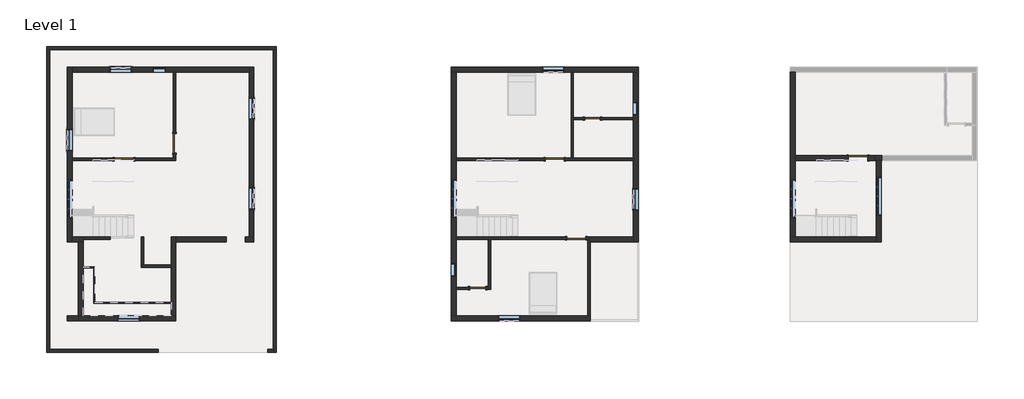
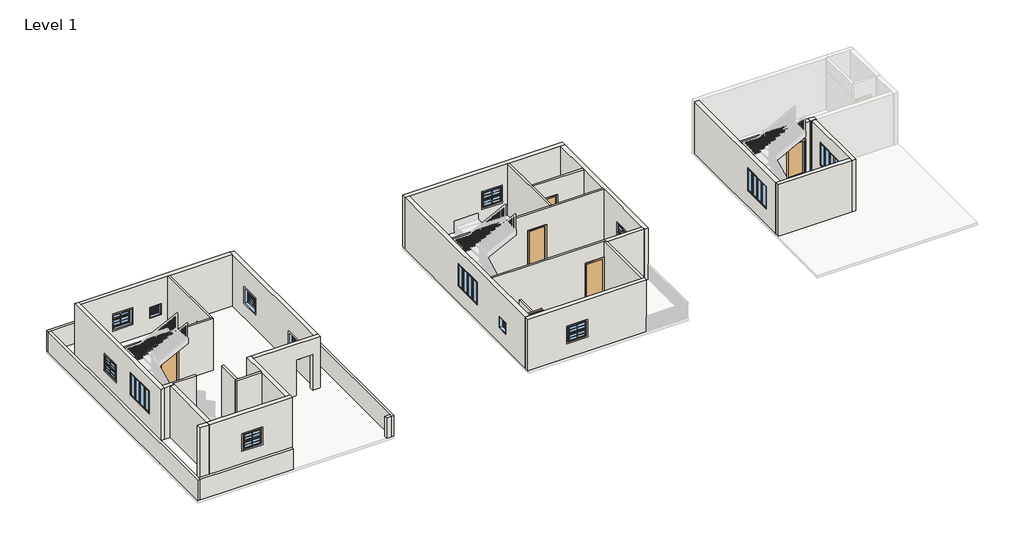
# One storey, part 1 of 8: 40 walls, 15 windows, 7 doors.
# Revit data of these elements (continued)
# Element 51 (IfcWindow, "Window-Awning-Double-Vertical : 41\" x 36\"")
#   Mark = "8"
#   Window Inset = 0' - 0"
#   Interior Wall Closure = 0' - 2 1/4"
#   Frame Extension = 0' - 0 1/4"
#   Exterior Wall Closure = 0' - 1 1/4"
#   Interior Trim Visibility = yes
#   Exterior Trim Visibility = yes
#   Phase Created = New Construction
#   Materials on its faces: "Wood - Stained", "Glass", "Clad - White"
# Element 52 (IfcWindow, "Window-Awning-Double-Vertical : 41\" x 36\"")
#   Mark = "9"
#   Window Inset = 0' - 0"
#   Interior Wall Closure = 0' - 2 1/4"
#   Frame Extension = 0' - 0 1/4"
#   Exterior Wall Closure = 0' - 1 1/4"
#   Interior Trim Visibility = yes
#   Exterior Trim Visibility = yes
#   Phase Created = New Construction
#   Materials on its faces: "Wood - Stained", "Glass", "Clad - White"
# Element 53 (IfcWindow, "Window-Awning-Double-Vertical : 41\" x 36\"")
#   Mark = "10"
#   Window Inset = 0' - 0"
#   Interior Wall Closure = 0' - 2 1/4"
#   Frame Extension = 0' - 0 1/4"
#   Exterior Wall Closure = 0' - 1 1/4"
#   Interior Trim Visibility = yes
#   Exterior Trim Visibility = yes
#   Phase Created = New Construction
#   Materials on its faces: "Wood - Stained", "Glass", "Clad - White"
# Element 54 (IfcWindow, "Window-Awning-Double-Vertical : 41\" x 36\"")
#   Mark = "11"
#   Window Inset = 0' - 0"
#   Interior Wall Closure = 0' - 2 1/4"
#   Frame Extension = 0' - 0 1/4"
#   Exterior Wall Closure = 0' - 1 1/4"
#   Interior Trim Visibility = yes
#   Exterior Trim Visibility = yes
#   Phase Created = New Construction
#   Materials on its faces: "Wood - Stained", "Glass", "Clad - White"
# Element 55 (IfcWindow, "Window-Awning-Double-Vertical : 41\" x 36\"")
#   Mark = "12"
#   Window Inset = 0' - 0"
#   Interior Wall Closure = 0' - 2 1/4"
#   Frame Extension = 0' - 0 1/4"
#   Exterior Wall Closure = 0' - 1 1/4"
#   Interior Trim Visibility = yes
#   Exterior Trim Visibility = yes
#   Phase Created = New Construction
#   Materials on its faces: "Wood - Stained", "Glass", "Clad - White"
# Element 56 (IfcWindow, "Window-Casement-Multi-Sash-Horizontal : 72\" x 53\"")
#   Mark = "1"
#   Window Inset = 0' - 0 5/8"
#   Frame Gap 3 = 0' - 1 83/128"
#   Frame Gap 2 = 0' - 0 5/8"
#   Phase Created = New Construction
#   Materials on its faces: "Metal - Aluminum", "Glass"
# Element 57 (IfcWindow, "Window-Casement-Multi-Sash-Horizontal : 72\" x 53\"")
#   Mark = "2"
#   Window Inset = 0' - 0 5/8"
#   Frame Gap 3 = 0' - 1 83/128"
#   Frame Gap 2 = 0' - 0 5/8"
#   Phase Created = New Construction
#   Materials on its faces: "Metal - Aluminum", "Glass"
# Element 58 (IfcWindow, "Window-Casement-Multi-Sash-Horizontal : 72\" x 53\"")
#   Mark = "3"
#   Window Inset = 0' - 0 5/8"
#   Frame Gap 3 = 0' - 1 83/128"
#   Frame Gap 2 = 0' - 0 5/8"
#   Phase Created = New Construction
#   Materials on its faces: "Metal - Aluminum", "Glass"
# Element 59 (IfcWindow, "Window-Casement-Multi-Sash-Horizontal : 72\" x 53\"")
#   Mark = "4"
#   Window Inset = 0' - 0 5/8"
#   Frame Gap 3 = 0' - 1 83/128"
#   Frame Gap 2 = 0' - 0 5/8"
#   Phase Created = New Construction
#   Materials on its faces: "Metal - Aluminum", "Glass"
# Element 60 (IfcWindow, "Window-Louvers : 24\" x 24\"")
#   Mark = "13"
#   Blade Width = 1' - 10 1/2"
#   Phase Created = New Construction
#   Materials on its faces: "Birch"
# Element 61 (IfcWindow, "Window-Louvers : 24\" x 24\"")
#   Mark = "14"
#   Blade Width = 1' - 10 1/2"
#   Phase Created = New Construction
#   Materials on its faces: "Birch"
# Element 62 (IfcWindow, "Window-Louvers : 24\" x 24\"")
#   Mark = "15"
#   Blade Width = 1' - 10 1/2"
#   Phase Created = New Construction
#   Materials on its faces: "Birch"
# Materials
#   "Door - Panel": class "Wood", colour RGB 210 159 95, transparency 0, Cost = 0
#   "Door - Frame": colour RGB 118 70 51, transparency 0, Cost = 0
#   "Wood - Stained": class "Wood", colour RGB 224 178 126, transparency 0, Cost = 0
#   "Glass": class "Glass", colour RGB 0 128 192, transparency 0.75, Description = "Soda Lime Glass", Cost = 0
#   "Clad - White": class "Wood", colour RGB 242 242 238, transparency 0, Cost = 0
#   "Metal - Aluminum": class "Metal", colour RGB 247 247 247, transparency 0
#   "Birch": class "Wood", colour RGB 224 178 126, transparency 0, Description = "Betula Alleghaniensis", Cost = 0
#   "Paint - Sienna": colour RGB 118 70 51, transparency 0, Cost = 0
#   "Default Wall": colour RGB 128 128 128, transparency 0, Cost = 0
#   "WOODEN I": class "Generic", colour RGB 120 120 120, transparency 0, Cost = 0
#   "1 wall": class "Glass", colour RGB 0 0 255, transparency 0.75, Cost = 0
#   "7f 678e": class "Generic", colour RGB 120 120 120, transparency 0, Cost = 0
#   "TILES": class "Generic", colour RGB 120 120 120, transparency 0, Cost = 0
